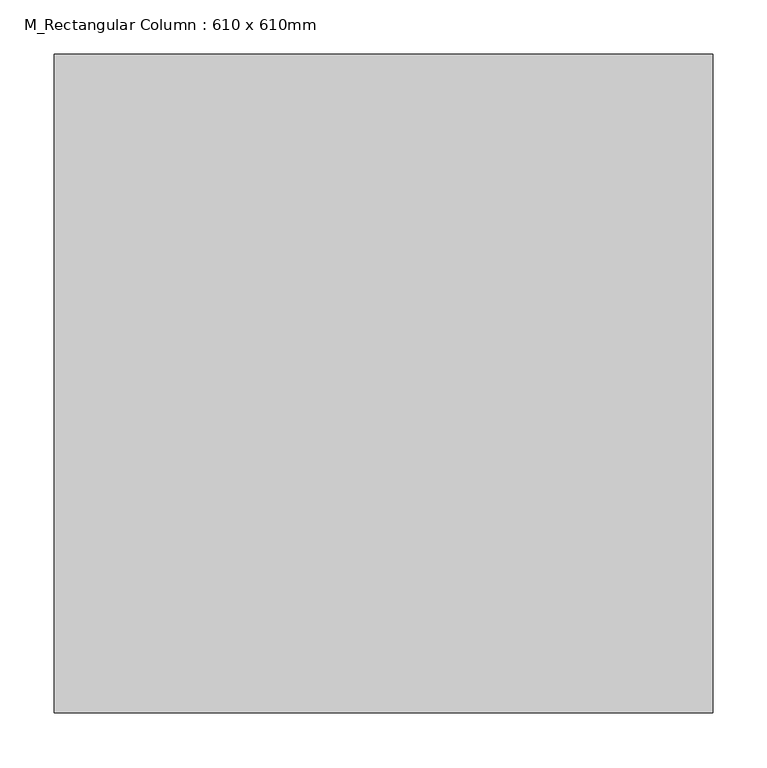
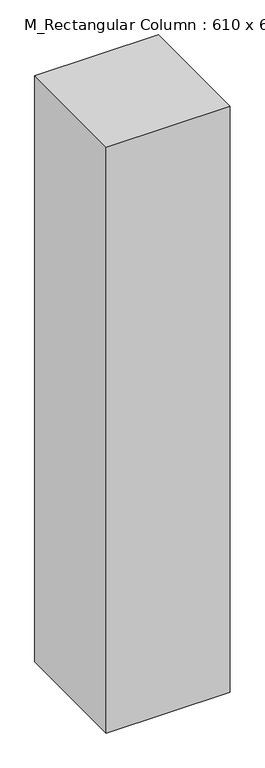
"""IFC4 building model written with IfcOpenShell, lengths in millimetres: column geometry, M_Rectangular Column : 610 x 610mm."""

from ifc_helpers import new_model, si_unit, origin, origin_with_axes, place, context, project, spatial, polyline, outline, extrude, source, transform, mapped, element, save


def m_rectangular_column_610_x_610mm_b887bf16(model_context):
    return source(origin(), model_context, "Body", "SweptSolid", [
        extrude(outline(polyline([(305.0, 305.0), (305.0, -305.0), (-305.0, -305.0), (-305.0, 305.0), (305.0, 305.0)])), origin_with_axes(), (0.0, 0.0, 1.0), 3048.0),
    ])


if __name__ == "__main__":
    model = new_model("IFC4")
    model_context = context("Model", 3, world=origin())
    ifc_project = project(units=[si_unit("LENGTHUNIT", "METRE", prefix="MILLI")], contexts=[model_context])
    site = spatial("IfcSite", under=ifc_project)
    building = spatial("IfcBuilding", under=site)
    placement = place(None, origin())
    m_rectangular_column_610_x_610mm_shape = m_rectangular_column_610_x_610mm_b887bf16(model_context)
    element("IfcColumn", 1, ObjectType="M_Rectangular Column : 610 x 610mm", at=placement, inside=building, context=model_context, shape_type="MappedRepresentation", body=[
        mapped(m_rectangular_column_610_x_610mm_shape, transform((0.0, 0.0, 0.0), x_axis=(1.0, 0.0, 0.0), y_axis=(0.0, 1.0, 0.0), z_axis=(0.0, 0.0, 1.0))),
    ])
    save(model, "model.ifc")

# Revit data of these elements
# Type "M_Rectangular Column : 610 x 610mm"
#   Depth = 610 mm
#   Offset Base = 0 mm
#   Offset Top = 0 mm
#   Width = 610 mm
#   Material = none
